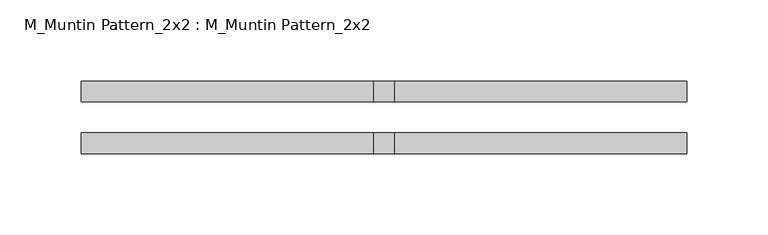
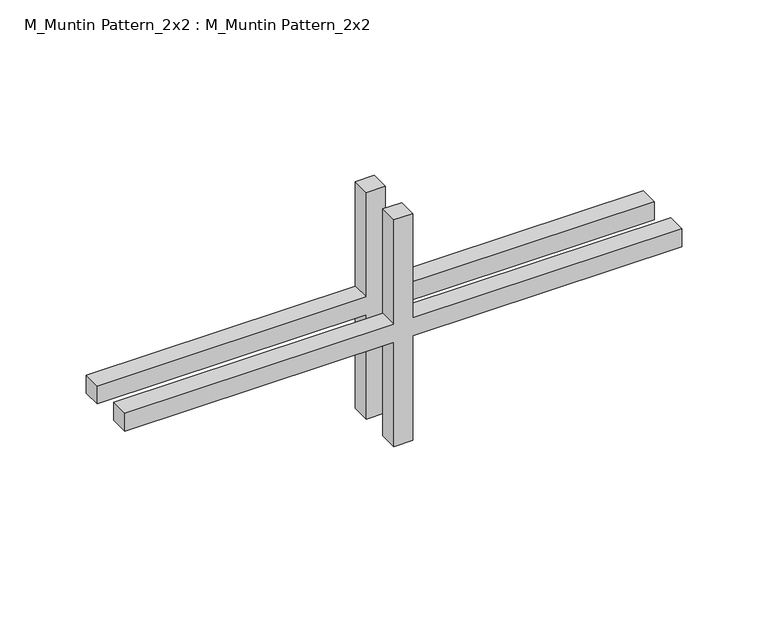
"""IFC4 building model written with IfcOpenShell, lengths in millimetres: proxy geometry, M_Muntin Pattern_2x2 : M_Muntin Pattern_2x2."""

from ifc_helpers import new_model, si_unit, frame, origin, place, context, project, spatial, polyline, outline, extrude, source, transform, mapped, element, save


def m_muntin_pattern_2x2_m_muntin_pattern_2x2_b257745b(model_context):
    return source(origin(), model_context, "Body", "SweptSolid", [
        extrude(outline(polyline([(86.5, -6.35), (86.5, -186.2666667), (73.8, -186.2666667), (73.8, -6.35), (0.0, -6.35), (0.0, 6.35), (73.8, 6.35), (73.8, 186.2666667), (86.5, 186.2666667), (86.5, 6.35), (160.3, 6.35), (160.3, -6.35), (86.5, -6.35)])), frame((0.0, 9.525, 0.0), z_axis=(0.0, 1.0, 0.0), x_axis=(0.0, 0.0, 1.0)), (0.0, 0.0, 1.0), 12.7),
        extrude(outline(polyline([(86.5, -6.35), (86.5, -186.2666667), (73.8, -186.2666667), (73.8, -6.35), (0.0, -6.35), (0.0, 6.35), (73.8, 6.35), (73.8, 186.2666667), (86.5, 186.2666667), (86.5, 6.35), (160.3, 6.35), (160.3, -6.35), (86.5, -6.35)])), frame((0.0, -22.225, 0.0), z_axis=(0.0, 1.0, 0.0), x_axis=(0.0, 0.0, 1.0)), (0.0, 0.0, 1.0), 12.7),
    ])


if __name__ == "__main__":
    model = new_model("IFC4")
    model_context = context("Model", 3, world=origin())
    ifc_project = project(units=[si_unit("LENGTHUNIT", "METRE", prefix="MILLI")], contexts=[model_context])
    site = spatial("IfcSite", under=ifc_project)
    building = spatial("IfcBuilding", under=site)
    placement = place(None, origin())
    m_muntin_pattern_2x2_m_muntin_pattern_2x2_shape = m_muntin_pattern_2x2_m_muntin_pattern_2x2_b257745b(model_context)
    element("IfcBuildingElementProxy", 1, Name="M_Muntin Pattern_2x2 : M_Muntin Pattern_2x2", ObjectType="M_Muntin Pattern_2x2 : M_Muntin Pattern_2x2", at=placement, inside=building, context=model_context, shape_type="MappedRepresentation", body=[
        mapped(m_muntin_pattern_2x2_m_muntin_pattern_2x2_shape, transform((0.0, 0.0, 0.0), x_axis=(1.0, 0.0, 0.0), y_axis=(0.0, 1.0, 0.0), z_axis=(0.0, 0.0, 1.0))),
    ])
    save(model, "model.ifc")

# Revit data of these elements
# Type "M_Muntin Pattern_2x2 : M_Muntin Pattern_2x2"
#   Width [instance default] = 3' - 11.24409"
#   Thickness = 0' - 0 1/2"
#   Height [instance default] = 3' - 11.24409"
#   Distance = 0' - 0 3/4"
#   Interior Material [instance default] = none
#   Exterior Material [instance default] = none
#   Default Elevation = 0
# Element 1 (IfcBuildingElementProxy, "M_Muntin Pattern_2x2 : M_Muntin Pattern_2x2")
#   Width = 1' - 2.66667"
#   Height = 0' - 6.31102"
#   Interior Material = Wood - Stained
#   Exterior Material = Clad - White
#   Materials on its faces: "Clad - White", "Wood - Stained"
# Materials
#   "Clad - White": class "Wood", colour RGB 242 242 238, transparency 0, Cost = 0
#   "Wood - Stained": class "Wood", colour RGB 224 178 126, transparency 0, Cost = 0
